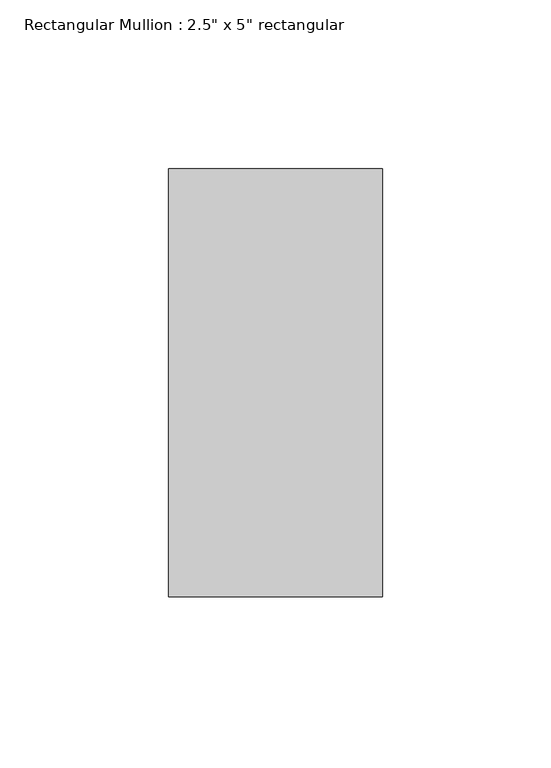
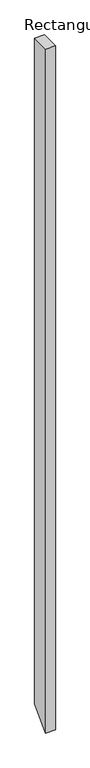
"""IFC4 building model written with IfcOpenShell, lengths in millimetres: member geometry."""

from ifc_helpers import new_model, si_unit, frame, origin, place, context, project, spatial, polyline, outline, extrude, source, transform, mapped, element, save


def member_41daa855(model_context):
    return source(origin(), model_context, "Body", "SweptSolid", [
        extrude(outline(polyline([(-63.5, 0.0), (63.5, 0.0), (63.5, -4658.2504165), (-63.5, -4785.2504165), (-63.5, 0.0)])), frame((-63.5, 0.0, 0.0), z_axis=(1.0, 0.0, 0.0), x_axis=(0.0, 1.0, 0.0)), (0.0, 0.0, 1.0), 63.5),
    ])


if __name__ == "__main__":
    model = new_model("IFC4")
    model_context = context("Model", 3, world=origin())
    ifc_project = project(units=[si_unit("LENGTHUNIT", "METRE", prefix="MILLI")], contexts=[model_context])
    site = spatial("IfcSite", under=ifc_project)
    building = spatial("IfcBuilding", under=site)
    placement = place(None, origin())
    member_shape = member_41daa855(model_context)
    element("IfcMember", 1, ObjectType="Rectangular Mullion : 2.5\" x 5\" rectangular", at=placement, inside=building, context=model_context, shape_type="MappedRepresentation", body=[
        mapped(member_shape, transform((0.0, 0.0, 0.0), x_axis=(1.0, 0.0, 0.0), y_axis=(0.0, 1.0, 0.0), z_axis=(0.0, 0.0, 1.0))),
    ])
    save(model, "model.ifc")

# Revit data of these elements
# Type "Rectangular Mullion : 2.5\" x 5\" rectangular"
#   built-in parameter 1007304 = 0.416667 (stored number, unit not read)
#   built-in parameter 1007301 = 0.104167 (stored number, unit not read)
#   built-in parameter 1007300 = 0.104167 (stored number, unit not read)
# Element 1 (IfcMember, "Rectangular Mullion : 2.5\" x 5\" rectangular")
#   Materials on its faces: "Aluminum"
# Materials
#   "Aluminum": class "Metal", colour RGB 247 247 247, transparency 0, Description = "Aluminum 6061", Cost = 0
